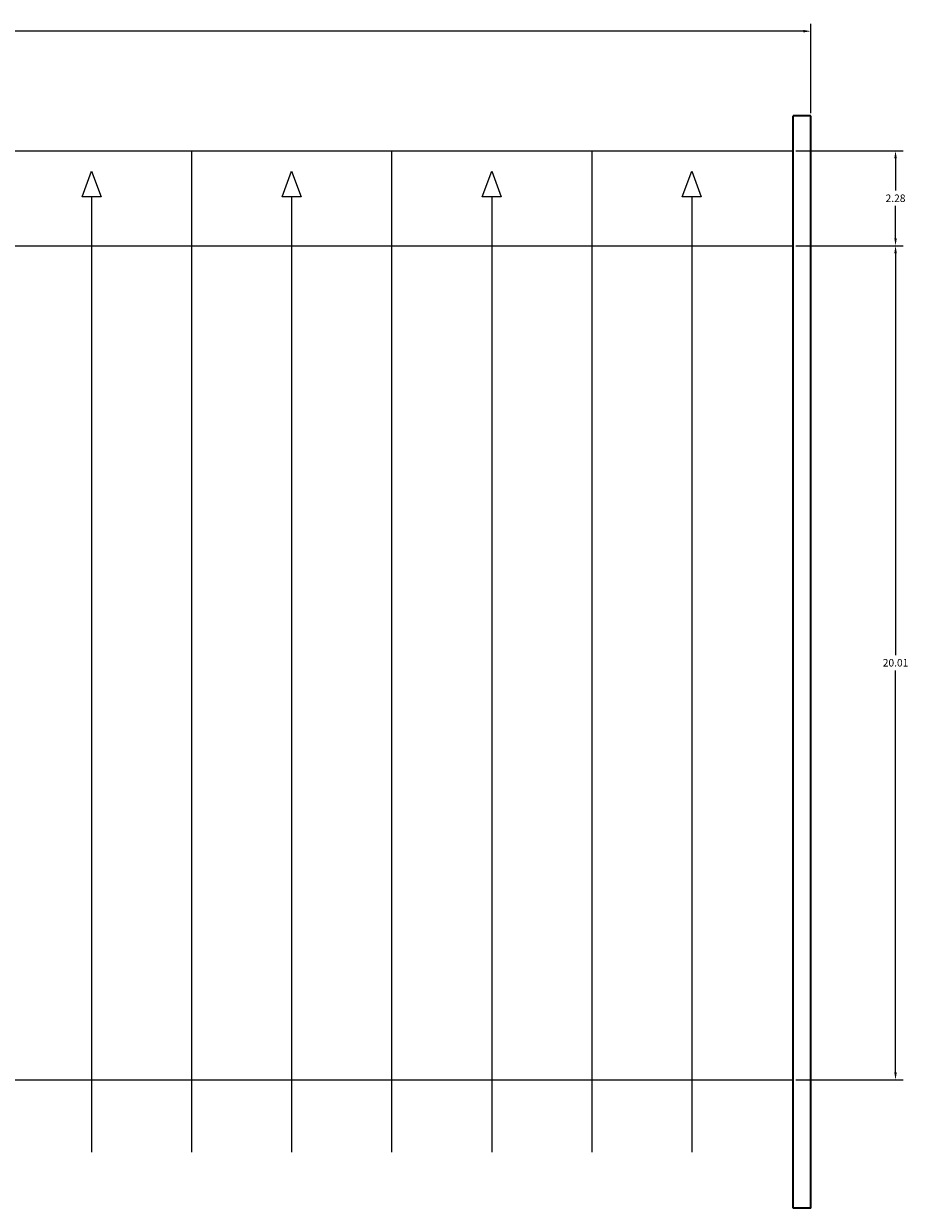
# Model space of a CAD drawing. Units: inches. Extents: x 756 to 915, y 488 to 695.
# Tile 16 of 25: x 791 to 812, y 629 to 658. Entities that reach past the tile are written whole.
import ezdxf

# ---------------------------------------------------------------- set-up
doc = ezdxf.new("R2010")
doc.units = ezdxf.units.IN
doc.header["$MEASUREMENT"] = 0
for name, color, linetype, lineweight in [('L-FENC-PCKT', 7, 'Continuous', 18), ('L-FENC-POST', 7, 'Continuous', 35), ('L-FENC-RAIL', 7, 'Continuous', 25), ('M-DIMS', 2, 'Continuous', 18)]:
    doc.layers.add(name, color=color, linetype=linetype, lineweight=lineweight)
doc.styles.get("Standard").update_dxf_attribs({"font": 'arial.ttf'})
doc.dimstyles.get("Standard").update_dxf_attribs({"dimtxt": 0.18, "dimasz": 0.18, "dimexe": 0.18, "dimexo": 0.0625, "dimgap": 0.09, "dimtad": 0, "dimtih": 1, "dimtoh": 1, "dimdec": 0, "dimzin": 0, "dimdsep": 46, "dimlunit": 3, "dimtxsty": 'Standard', "dimcen": 0.09, "dimadec": 0, "dimazin": 0, "dimtfac": 1, "dimtdec": 0, "dimtofl": 0, "dimtmove": 0, "dimatfit": 3, "dimfxl": 1, "dimtolj": 1, "dimtzin": 0, "dimarcsym": 0})

# ---------------------------------------------------------------- blocks, each defined once
blk = doc.blocks.new('FENCE-POST-RIGHT')
for p, q in [((0, 26.207), (0, 0)), ((0, 26.207), (0.427, 26.207)), ((0.427, 26.207), (0.427, 0)), ((0, 0), (0.427, 0))]:
    blk.add_line(p, q)
blk = doc.blocks.new('PICKET-SPEAR-LOW')
blk.add_line((0.228, 22.916), (0.228, 0))
blk.add_lwpolyline([(0.228, 22.916), (0, 22.916), (0.228, 23.528), (0.455, 22.916)], close=True)
blk = doc.blocks.new('*D32')
at = {"layer": 'Defpoints', "color": 0, "transparency": 16777216}
for p in [(809.674, 657.541), (770.216, 655.511), (809.674, 655.511)]:
    blk.add_point(p, dxfattribs=at)
at = {"layer": 'M-DIMS', "color": 0, "lineweight": -2, "transparency": 16777216}
for p, q in [((770.216, 655.574), (770.216, 657.721)), ((809.674, 655.574), (809.674, 657.721)), ((770.396, 657.541), (789.551, 657.541)), ((809.494, 657.541), (790.338, 657.541))]:
    blk.add_line(p, q, dxfattribs=at)
at = {"layer": 'M-DIMS', "color": 0, "transparency": 16777216}
for points in [[(770.396, 657.571), (770.396, 657.511), (770.216, 657.541)], [(809.494, 657.571), (809.494, 657.511), (809.674, 657.541)]]:
    blk.add_solid(points, dxfattribs=at)
at = {"layer": 'M-DIMS', "color": 0, "transparency": 16777216, "insert": (789.945, 657.541), "char_height": 0.18, "attachment_point": 5}
blk.add_mtext('\\A1;39.46', dxfattribs=at)
blk = doc.blocks.new('*D35')
at = {"layer": 'Defpoints', "color": 0, "transparency": 16777216}
for p in [(809.247, 652.396), (811.704, 652.396), (809.247, 632.386)]:
    blk.add_point(p, dxfattribs=at)
at = {"layer": 'M-DIMS', "color": 0, "lineweight": -2, "transparency": 16777216}
for p, q in [((809.31, 652.396), (811.884, 652.396)), ((811.704, 652.216), (811.704, 642.573)), ((811.704, 632.566), (811.704, 642.209)), ((809.31, 632.386), (811.884, 632.386))]:
    blk.add_line(p, q, dxfattribs=at)
at = {"layer": 'M-DIMS', "color": 0, "transparency": 16777216}
for points in [[(811.674, 652.216), (811.734, 652.216), (811.704, 652.396)], [(811.674, 632.566), (811.734, 632.566), (811.704, 632.386)]]:
    blk.add_solid(points, dxfattribs=at)
at = {"layer": 'M-DIMS', "color": 0, "transparency": 16777216, "insert": (811.704, 642.391), "char_height": 0.18, "attachment_point": 5}
blk.add_mtext('\\A1;20.01', dxfattribs=at)
blk = doc.blocks.new('*D36')
at = {"layer": 'Defpoints', "color": 0, "transparency": 16777216}
for p in [(809.247, 654.673), (811.704, 654.673), (809.247, 652.396)]:
    blk.add_point(p, dxfattribs=at)
at = {"layer": 'M-DIMS', "color": 0, "lineweight": -2, "transparency": 16777216}
for p, q in [((809.31, 654.673), (811.884, 654.673)), ((811.704, 654.493), (811.704, 653.716)), ((811.704, 652.576), (811.704, 653.352)), ((809.31, 652.396), (811.884, 652.396))]:
    blk.add_line(p, q, dxfattribs=at)
at = {"layer": 'M-DIMS', "color": 0, "transparency": 16777216}
for points in [[(811.674, 654.493), (811.734, 654.493), (811.704, 654.673)], [(811.674, 652.576), (811.734, 652.576), (811.704, 652.396)]]:
    blk.add_solid(points, dxfattribs=at)
at = {"layer": 'M-DIMS', "color": 0, "transparency": 16777216, "insert": (811.704, 653.534), "char_height": 0.18, "attachment_point": 5}
blk.add_mtext('\\A1;2.28', dxfattribs=at)

msp = doc.modelspace()

# ---------------------------------------------------------------- linework, layer by layer
at = {"layer": 'L-FENC-PCKT'}
for p, q in [((794.8139, 654.6726), (794.8139, 630.6539)), ((799.6138, 654.6726), (799.6138, 630.6539)), ((804.4136, 654.6726), (804.4136, 630.6539))]:
    msp.add_line(p, q, dxfattribs=at)
at = {"layer": 'L-FENC-RAIL'}
for p, q in [((770.6423, 654.6726), (809.2471, 654.6726)), ((770.6423, 652.3962), (809.2471, 652.3962)), ((770.6423, 632.386), (809.2471, 632.386))]:
    msp.add_line(p, q, dxfattribs=at)

# ---------------------------------------------------------------- block references
at = {"layer": 'L-FENC-PCKT'}
for p in [(792.1863, 630.6543), (796.9861, 630.6543), (801.7859, 630.6543), (806.5858, 630.6543)]:
    msp.add_blockref('PICKET-SPEAR-LOW', p, dxfattribs=at)
at = {"layer": 'L-FENC-POST', "rotation": 180}
msp.add_blockref('FENCE-POST-RIGHT', (809.6739, 655.5112), dxfattribs=at)

# ---------------------------------------------------------------- dimensions: what is measured, and where the dimension line sits
at = {"layer": 'M-DIMS'}
dim = msp.add_linear_dim(base=(809.6738, 657.5412), p1=(770.2156, 655.5112), p2=(809.6738, 655.5112), dimstyle='Standard', override={"dimdec": 2, "dimlfac": 1, "dimrnd": 0, "dimzin": 0, "dimdsep": 46, "dimlunit": 2}, dxfattribs=at)
dim.commit()
dim.dimension.update_dxf_attribs({"geometry": '*D32', "text_midpoint": (789.9447, 657.5412)})
for base, p1, p2, picture, middle in [((811.7038, 654.6726), (809.2471, 652.3962), (809.2471, 654.6726), '*D36', (811.7038, 653.5344)), ((811.7038, 652.3962), (809.2471, 632.386), (809.2471, 652.3962), '*D35', (811.7038, 642.3911))]:
    dim = msp.add_linear_dim(base=base, p1=p1, p2=p2, angle=90, dimstyle='Standard', override={"dimdec": 2, "dimlfac": 1, "dimrnd": 0, "dimzin": 0, "dimdsep": 46, "dimlunit": 2}, dxfattribs=at)
    dim.commit()
    dim.dimension.update_dxf_attribs({"geometry": picture, "text_midpoint": middle})

doc.saveas('drawing.dxf')
